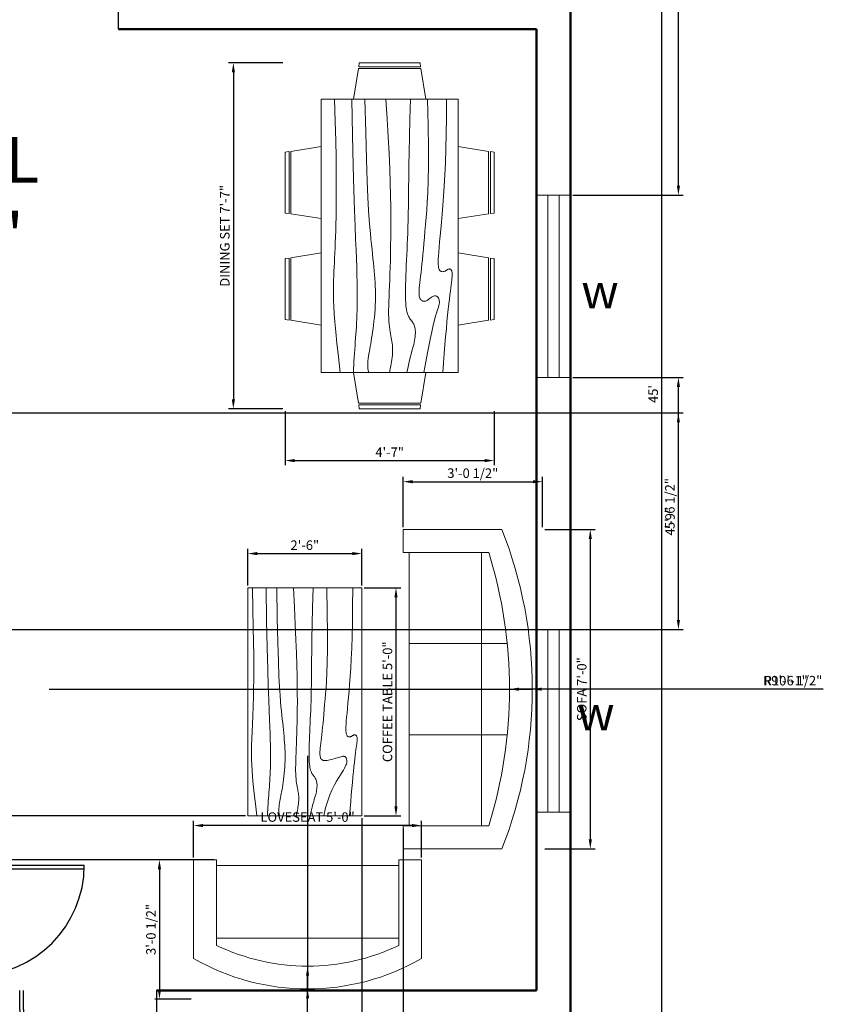
# Model space of a CAD drawing. Units: inches. Extents: x 1962 to 2423, y 2693 to 3296.
# Tile 3 of 4: x 2212 to 2423, y 2833 to 3092. Entities that reach past the tile are written whole.
import ezdxf

# ---------------------------------------------------------------- set-up
doc = ezdxf.new("R2010")
doc.units = ezdxf.units.IN
for name, color, linetype, lineweight in [('A-ANNO-DIMS', 2, 'Continuous', 18), ('A-ANNO-TEXT', 3, 'Continuous', 18), ('A-AREA-IDEN', 7, 'Continuous', 25), ('A-DOOR', 3, 'Continuous', 25), ('A-FURN', 8, 'Continuous', 18), ('A-GLAZ', 4, 'Continuous', 18), ('A-WALL', 7, 'Continuous', 50)]:
    doc.layers.add(name, color=color, linetype=linetype, lineweight=lineweight)
doc.styles.get("Standard").update_dxf_attribs({"font": 'arial.ttf'})
doc.dimstyles.new('ISO-25', dxfattribs={"dimtxt": 2.5, "dimasz": 2.5, "dimexe": 1.25, "dimexo": 0.625, "dimtad": 1, "dimdec": 0, "dimlunit": 3, "dimtxsty": 'Standard', "dimcen": 2.5, "dimadec": 0, "dimazin": 0, "dimtfac": 1, "dimtdec": 0, "dimtmove": 0, "dimatfit": 3, "dimfxl": 1, "dimarcsym": 0})

# ---------------------------------------------------------------- blocks, each defined once
blk = doc.blocks.new('Sofa - Roundback 7 ft.')
for p, q in [((-12.00002, -32.4421), (-12.00003, -6.5971)), ((11.99997, -32.4421), (11.99998, -6.5971)), ((-36.000027, -34), (-36.000027, -11.4696)), ((35.99998, -34), (35.99998, -11.4696)), ((-35.999844, -13.3819), (35.9998, -13.3819)), ((-36.000027, -32.4421), (35.99998, -32.4421))]:
    blk.add_line(p, q)
for points in [[(-36.000027, -34), (-42.000027, -34), (-42.000027, -8)], [(41.99998, -8), (41.99998, -34), (35.99998, -34)]]:
    blk.add_lwpolyline(points)
for centre, radius, start, end in [((0, -114.25), 114.25, 68.43141, 111.5686), ((-0.00001, -127.1968), 121.1968, 72.72033, 107.2797)]:
    blk.add_arc(centre, radius, start, end)
blk = doc.blocks.new('Sofa - Roundback Loveseat 5 ft.')
for p, q in [((0, -32.44198), (0, -5.99998)), ((-24, -33.99998), (-24, -11.46958)), ((24.00004, -33.99998), (24.00004, -11.46958)), ((-23.9998, -13.38178), (23.99986, -13.38178)), ((-24, -32.44198), (24.00004, -32.44198))]:
    blk.add_line(p, q)
for points in [[(-24, -33.99998), (-30, -33.99998), (-30, -7.99998)], [(30.00004, -7.99998), (30.00004, -33.99998), (24.00004, -33.99998)]]:
    blk.add_lwpolyline(points)
for centre, radius, start, end in [((0, -60.24998), 60.24998, 60.13715, 119.8628), ((0, -61.38438), 55.38444, 64.32083, 115.6792)]:
    blk.add_arc(centre, radius, start, end)
blk = doc.blocks.new('Table - Rectangular Woodgrain 60 x 30 in.')
for p, q in [((0, 0), (0, -30)), ((60, 0), (0, 0)), ((60, -30), (60, 0)), ((0, -30), (60, -30))]:
    blk.add_line(p, q)
for points in [[(0, -2.4), (4.8155, -2.418), (9.0302, -2.4688), (12.709, -2.5477), (15.9167, -2.65), (18.7181, -2.7711), (21.1781, -2.9063), (23.3616, -3.0508), (25.3333, -3.2), (27.1477, -3.3495), (28.8172, -3.4958), (30.3437, -3.636), (31.7291, -3.7667), (32.9756, -3.8849), (34.0849, -3.9875), (35.059, -4.0714), (35.9, -4.1334), (36.6114, -4.1711), (37.2041, -4.1854), (37.6906, -4.1779), (38.0833, -4.15), (38.3948, -4.1034), (38.6375, -4.0396), (38.8239, -3.9602), (38.9666, -3.8667), (39.0764, -3.7608), (39.1573, -3.6448), (39.2116, -3.521), (39.2416, -3.3917), (39.2498, -3.2593), (39.2385, -3.1261), (39.21, -2.9944), (39.1666, -2.8667), (39.111, -2.7447), (39.0468, -2.6281), (38.978, -2.5163), (38.9083, -2.4083), (38.8418, -2.3035), (38.7823, -2.201), (38.7337, -2.1001), (38.7, -2), (38.6844, -1.9003), (38.6875, -1.8021), (38.7094, -1.707), (38.75, -1.6167), (38.8094, -1.5326), (38.8875, -1.4563), (38.9844, -1.3893), (39.1, -1.3333), (39.2351, -1.2896), (39.3937, -1.2583), (39.5804, -1.2396), (39.8, -1.2333), (40.057, -1.2396), (40.3562, -1.2583), (40.7023, -1.2896), (41.1, -1.3333), (41.5547, -1.3895), (42.0755, -1.4573), (42.6721, -1.5361), (43.3542, -1.625), (44.1316, -1.7233), (45.014, -1.8302), (46.0114, -1.9449), (47.1333, -2.0667), (48.3862, -2.1947), (49.7625, -2.3281), (51.2513, -2.4663), (52.8416, -2.6083), (54.5226, -2.7535), (56.2833, -2.9011), (58.1127, -3.0501), (60, -3.2)], [(0, -9.2), (6.5759, -9.0858), (11.9385, -9.0365), (16.2527, -9.0418), (19.6833, -9.0917), (22.3952, -9.1759), (24.5531, -9.2844), (26.322, -9.4069), (27.8666, -9.5333), (29.3241, -9.6553), (30.7203, -9.7719), (32.0532, -9.8837), (33.3208, -9.9917), (34.5213, -10.0965), (35.6526, -10.199), (36.7128, -10.2999), (37.7, -10.4), (38.6129, -10.4996), (39.4531, -10.5969), (40.223, -10.6895), (40.925, -10.775), (41.5613, -10.8512), (42.1344, -10.9156), (42.6465, -10.966), (43.1, -11), (43.4976, -11.0158), (43.8437, -11.0136), (44.143, -10.9942), (44.4, -10.9583), (44.6195, -10.9069), (44.8062, -10.8406), (44.9648, -10.7603), (45.1, -10.6667), (45.2155, -10.5598), (45.3114, -10.4365), (45.3871, -10.2929), (45.4416, -10.125), (45.4743, -9.929), (45.4844, -9.7011), (45.4709, -9.4371), (45.4333, -9.1333), (45.3716, -8.7883), (45.2896, -8.4104), (45.1919, -8.0107), (45.0833, -7.6), (44.9685, -7.1893), (44.8521, -6.7896), (44.7388, -6.4117), (44.6333, -6.0667), (44.54, -5.7628), (44.4614, -5.4979), (44.4001, -5.2675), (44.3583, -5.0667), (44.3384, -4.8909), (44.3427, -4.7354), (44.3736, -4.5956), (44.4333, -4.4667), (44.5236, -4.3453), (44.6427, -4.2333), (44.7884, -4.1339), (44.9583, -4.05), (45.1501, -3.9849), (45.3614, -3.9417), (45.59, -3.9234), (45.8333, -3.9333), (46.0915, -3.9749), (46.3734, -4.0531), (46.6906, -4.1736), (47.0542, -4.3417), (47.4756, -4.5629), (47.9661, -4.8427), (48.5372, -5.1866), (49.2, -5.6), (49.9676, -6.0844), (50.8594, -6.625), (51.8965, -7.2031), (53.1, -7.8), (54.491, -8.3969), (56.0906, -8.975), (57.9199, -9.5156), (60, -10)], [(0, -12.8), (5.1847, -12.9322), (9.6213, -13.0323), (13.3963, -13.1059), (16.5958, -13.1583), (19.3063, -13.1952), (21.614, -13.2219), (23.6054, -13.2439), (25.3666, -13.2667), (26.9728, -13.2947), (28.4531, -13.3281), (29.8256, -13.3663), (31.1083, -13.4083), (32.3191, -13.4535), (33.476, -13.501), (34.597, -13.5501), (35.7, -13.6), (36.7984, -13.6497), (37.8875, -13.6979), (38.9578, -13.743), (40, -13.7833), (41.0047, -13.8174), (41.9625, -13.8438), (42.864, -13.8607), (43.7, -13.8667), (44.4631, -13.8604), (45.1552, -13.8417), (45.7801, -13.8104), (46.3416, -13.7667), (46.8439, -13.7104), (47.2906, -13.6417), (47.6858, -13.5604), (48.0333, -13.4667), (48.3375, -13.3608), (48.6042, -13.2448), (48.8396, -13.121), (49.05, -12.9917), (49.2417, -12.8593), (49.4208, -12.7261), (49.5937, -12.5944), (49.7667, -12.4667), (49.9452, -12.3451), (50.1323, -12.2313), (50.3303, -12.1268), (50.5416, -12.0333), (50.7686, -11.9524), (51.0135, -11.8854), (51.2788, -11.8341), (51.5666, -11.8), (51.8785, -11.7843), (52.2116, -11.7865), (52.562, -11.8059), (52.926, -11.8417), (53.2998, -11.8931), (53.6795, -11.9594), (54.0614, -12.0397), (54.4416, -12.1333), (54.8223, -12.2401), (55.2293, -12.3625), (55.6942, -12.5037), (56.2489, -12.6667), (56.9251, -12.8547), (57.7545, -13.0708), (58.7689, -13.3182), (60, -13.6)], [(0, -18), (5.124, -17.7273), (9.6609, -17.5057), (13.6705, -17.3303), (17.2125, -17.1958), (20.3467, -17.0973), (23.1328, -17.0297), (25.6307, -16.9878), (27.9, -16.9667), (29.9928, -16.9617), (31.9302, -16.9703), (33.7254, -16.9907), (35.3917, -17.0208), (36.9423, -17.0588), (38.3906, -17.1026), (39.7499, -17.1503), (41.0333, -17.2), (42.2519, -17.2496), (43.4073, -17.2969), (44.4986, -17.3395), (45.525, -17.375), (46.4858, -17.4012), (47.3802, -17.4156), (48.2074, -17.416), (48.9667, -17.4), (49.6583, -17.3662), (50.2872, -17.3167), (50.8595, -17.2547), (51.3812, -17.1833), (51.8584, -17.1057), (52.2971, -17.025), (52.7034, -16.9443), (53.0833, -16.8667), (53.443, -16.7951), (53.789, -16.7313), (54.128, -16.6768), (54.4666, -16.6334), (54.8115, -16.6024), (55.1693, -16.5854), (55.5465, -16.5841), (55.95, -16.6), (56.3828, -16.6337), (56.8346, -16.6823), (57.2915, -16.7418), (57.7396, -16.8084), (58.165, -16.878), (58.5539, -16.9469), (58.8924, -17.0111), (59.1666, -17.0667), (59.3679, -17.1107), (59.5078, -17.1438), (59.6032, -17.1675), (59.6708, -17.1833), (59.7275, -17.193), (59.7901, -17.1979), (59.8753, -17.1998), (60, -17.2)], [(0, -22.4), (8.0098, -22.2501), (14.4094, -22.1011), (19.4168, -21.9535), (23.25, -21.8083), (26.1269, -21.6663), (28.2656, -21.5281), (29.884, -21.3947), (31.2, -21.2667), (32.3967, -21.1448), (33.5172, -21.0292), (34.5697, -20.9198), (35.5625, -20.8167), (36.5037, -20.7198), (37.4015, -20.6292), (38.2642, -20.5448), (39.1, -20.4667), (39.9164, -20.3951), (40.7187, -20.3313), (41.5117, -20.2768), (42.3, -20.2333), (43.0883, -20.2024), (43.8812, -20.1854), (44.6836, -20.1841), (45.5, -20.2), (46.3328, -20.234), (47.1747, -20.2844), (48.0163, -20.3488), (48.8479, -20.425), (49.66, -20.5106), (50.4429, -20.6031), (51.1872, -20.7004), (51.8833, -20.8), (52.5246, -20.8999), (53.1166, -20.9995), (53.6681, -21.0983), (54.1875, -21.1958), (54.6834, -21.2919), (55.1646, -21.3859), (55.6394, -21.4777), (56.1167, -21.5667), (56.6028, -21.6515), (57.0961, -21.7266), (57.5929, -21.7852), (58.0896, -21.8208), (58.5823, -21.8268), (59.0674, -21.7964), (59.5412, -21.723), (60, -21.6)], [(0, -25.2), (8.6355, -25.0504), (15.7026, -24.9031), (21.4049, -24.7606), (25.9458, -24.625), (29.529, -24.4988), (32.3578, -24.3844), (34.6359, -24.284), (36.5667, -24.2), (38.3213, -24.1341), (39.9417, -24.0854), (41.437, -24.0523), (42.8167, -24.0333), (44.0901, -24.0268), (45.2667, -24.0313), (46.3557, -24.0451), (47.3667, -24.0667), (48.309, -24.0947), (49.1928, -24.1287), (50.0284, -24.168), (50.826, -24.2125), (51.5959, -24.2617), (52.3483, -24.3151), (53.0935, -24.3725), (53.8417, -24.4334), (54.6009, -24.497), (55.3699, -24.561), (56.1454, -24.6226), (56.9239, -24.6792), (57.7021, -24.7279), (58.4764, -24.7662), (59.2435, -24.7911), (60, -24.8)], [(0, -28.8), (5.6867, -28.6681), (10.45, -28.5698), (14.407, -28.5012), (17.675, -28.4584), (20.3711, -28.4374), (22.6125, -28.4344), (24.5164, -28.4455), (26.2, -28.4667), (27.762, -28.4947), (29.2276, -28.5281), (30.6033, -28.5663), (31.8958, -28.6084), (33.1118, -28.6535), (34.2578, -28.7011), (35.3405, -28.7501), (36.3666, -28.8), (37.3443, -28.8497), (38.288, -28.8974), (39.2137, -28.9412), (40.1375, -28.9792), (41.0753, -29.0093), (42.0432, -29.0297), (43.0572, -29.0384), (44.1333, -29.0333), (45.2936, -29.0114), (46.5843, -28.9641), (48.0579, -28.8816), (49.7666, -28.7542), (51.7629, -28.5721), (54.0989, -28.3255), (56.8272, -28.0048), (60, -27.6)]]:
    blk.add_lwpolyline(points)
blk = doc.blocks.new('Dining Set - 36 x 72 in.')
for p, q in [((-22.2343, 26.00059), (-23.4847, 17.99762)), ((-22.2304, 26), (-5.7608, 26)), ((-22, 27.5), (-22.1562, 26.50042)), ((-5.8416, 26.5), (-22.1534, 26.5)), ((-22, 27.5), (-6, 27.5)), ((-5.8437, 26.49966), (-6, 27.5)), ((-4.5152, 17.99762), (-5.7655, 25.99926)), ((5.7657, 26.00059), (4.5153, 17.99762)), ((5.7696, 26), (22.2392, 26)), ((6, 27.5), (5.8438, 26.50042)), ((22.1584, 26.5), (5.8466, 26.5)), ((6, 27.5), (22, 27.5)), ((22.1563, 26.49966), (22, 27.5)), ((23.4848, 17.99762), (22.2345, 25.99926)), ((36, 18), (-36, 18)), ((-36, 18), (-36, -18)), ((36, -18), (36, 18)), ((-45.5, 8), (-44.5004, 8.15617)), ((-45.5, 8), (-45.5, -8)), ((-44.5, -8.15843), (-44.5, 8.15338)), ((-44.0006, 8.23428), (-35.9976, 9.48474)), ((-44, 8.23041), (-44, -8.23915)), ((44.0006, 8.23428), (35.9976, 9.48474)), ((44, 8.23041), (44, -8.23915)), ((44.5, -8.15843), (44.5, 8.15338)), ((45.5, 8), (44.5005, 8.15617)), ((45.5, 8), (45.5, -8)), ((-44.4997, -8.15631), (-45.5, -8)), ((-35.9976, -9.48476), (-43.9993, -8.2345)), ((35.9976, -9.48476), (43.9993, -8.2345)), ((44.4997, -8.15631), (45.5, -8)), ((-36, -18), (36, -18)), ((-22.2343, -26.0006), (-23.4847, -17.99762)), ((-4.5152, -17.99762), (-5.7655, -25.99928)), ((5.7657, -26.0006), (4.5153, -17.99762)), ((23.4848, -17.99762), (22.2345, -25.99928)), ((-22.2304, -26), (-5.7608, -26)), ((-22, -27.5), (-22.1562, -26.50044)), ((-5.8416, -26.5), (-22.1534, -26.5)), ((-22, -27.5), (-6, -27.5)), ((-5.8437, -26.49967), (-6, -27.5)), ((5.7696, -26), (22.2392, -26)), ((6, -27.5), (5.8438, -26.50044)), ((22.1584, -26.5), (5.8466, -26.5)), ((6, -27.5), (22, -27.5)), ((22.1563, -26.49967), (22, -27.5))]:
    blk.add_line(p, q)
for points in [[(-36, 15), (-31.1772, 14.97754), (-26.8079, 14.91406), (-22.8538, 14.81543), (-19.276, 14.6875), (-16.0362, 14.53613), (-13.0957, 14.36718), (-10.4159, 14.18652), (-7.9583, 14), (-5.6904, 13.81315), (-3.6035, 13.63021), (-1.6954, 13.45508), (0.0365, 13.29166), (1.5945, 13.14388), (2.9811, 13.01562), (4.1988, 12.9108), (5.25, 12.83333), (6.1393, 12.78613), (6.8802, 12.76823), (7.4883, 12.77767), (7.9792, 12.8125), (8.3685, 12.87077), (8.6719, 12.95052), (8.9049, 13.0498), (9.0833, 13.16666), (9.2205, 13.29899), (9.3216, 13.44401), (9.3895, 13.59879), (9.4271, 13.76041), (9.4373, 13.92594), (9.4232, 14.09245), (9.3875, 14.257), (9.3333, 14.41666), (9.2638, 14.56917), (9.1836, 14.71484), (9.0975, 14.85465), (9.0104, 14.98958), (8.9272, 15.1206), (8.8529, 15.2487), (8.7922, 15.37483), (8.75, 15.5), (8.7305, 15.62467), (8.7344, 15.74739), (8.7617, 15.86621), (8.8125, 15.97916), (8.8867, 16.08431), (8.9844, 16.17968), (9.1055, 16.26334), (9.25, 16.33333), (9.4189, 16.38802), (9.6172, 16.42708), (9.8506, 16.45052), (10.125, 16.45833), (10.4463, 16.45052), (10.8203, 16.42708), (11.2529, 16.38802), (11.75, 16.33333), (12.3184, 16.26318), (12.9694, 16.17838), (13.7151, 16.07991), (14.5677, 15.96875), (15.5395, 15.84586), (16.6426, 15.71224), (17.8893, 15.56884), (19.2917, 15.41666), (20.859, 15.25667), (22.5879, 15.08984), (24.4721, 14.91715), (26.5052, 14.73958), (28.6809, 14.5581), (30.9929, 14.3737), (33.4347, 14.18733), (36, 14)], [(-36, 10), (-28.9766, 10.14274), (-23.1725, 10.20442), (-18.4241, 10.19775), (-14.5677, 10.13541), (-11.4399, 10.03011), (-8.877, 9.89453), (-6.7154, 9.74137), (-4.7917, 9.58333), (-2.9698, 9.43082), (-1.2246, 9.28515), (0.4415, 9.14534), (2.026, 9.01041), (3.5266, 8.87939), (4.9408, 8.7513), (6.266, 8.62516), (7.5, 8.5), (8.6411, 8.37549), (9.6914, 8.2539), (10.6538, 8.13818), (11.5312, 8.03125), (12.3267, 7.93603), (13.043, 7.85547), (13.6831, 7.79248), (14.25, 7.75), (14.7471, 7.7303), (15.1797, 7.73307), (15.5537, 7.75732), (15.875, 7.80208), (16.1494, 7.86637), (16.3828, 7.94922), (16.5811, 8.04964), (16.75, 8.16666), (16.8944, 8.29915), (17.0143, 8.44531), (17.1089, 8.60319), (17.1771, 8.77083), (17.218, 8.94629), (17.2305, 9.1276), (17.2137, 9.31282), (17.1667, 9.5), (17.0895, 9.6875), (16.987, 9.875), (16.8649, 10.0625), (16.7292, 10.25), (16.5856, 10.4375), (16.4401, 10.625), (16.2985, 10.8125), (16.1667, 11), (16.05, 11.18733), (15.9518, 11.3737), (15.8752, 11.5581), (15.8229, 11.73958), (15.798, 11.91715), (15.8034, 12.08984), (15.842, 12.25667), (15.9167, 12.41666), (16.0295, 12.56836), (16.1784, 12.70833), (16.3605, 12.83268), (16.5729, 12.9375), (16.8127, 13.01888), (17.0768, 13.07291), (17.3625, 13.0957), (17.6667, 13.08333), (17.9894, 13.03312), (18.3418, 12.94726), (18.7382, 12.82918), (19.1927, 12.68229), (19.7195, 12.51001), (20.3327, 12.31575), (21.0465, 12.10294), (21.875, 11.875), (22.8357, 11.63354), (23.959, 11.37304), (25.2786, 11.08618), (26.8282, 10.76562), (28.6414, 10.40405), (30.752, 9.99414), (33.1936, 9.52856), (36, 9)], [(-36, 5.5), (-30.7157, 5.3348), (-26.069, 5.20963), (-21.9946, 5.11767), (-18.4271, 5.05208), (-15.3009, 5.00602), (-12.5508, 4.97265), (-10.1112, 4.94515), (-7.9167, 4.91666), (-5.909, 4.88167), (-4.0586, 4.83984), (-2.3429, 4.79215), (-0.7396, 4.73958), (0.7739, 4.6831), (2.22, 4.6237), (3.6213, 4.56233), (5, 4.5), (6.373, 4.43782), (7.7344, 4.3776), (9.0723, 4.32129), (10.375, 4.27083), (11.6309, 4.22819), (12.8281, 4.19531), (13.9551, 4.17415), (15, 4.16666), (15.954, 4.17448), (16.819, 4.19791), (17.6001, 4.23698), (18.3021, 4.29166), (18.9299, 4.36198), (19.4883, 4.44791), (19.9823, 4.54948), (20.4167, 4.66666), (20.7969, 4.79899), (21.1302, 4.94401), (21.4245, 5.09879), (21.6875, 5.26041), (21.9271, 5.42594), (22.1511, 5.59245), (22.3672, 5.757), (22.5834, 5.91666), (22.8065, 6.06868), (23.0404, 6.21093), (23.2879, 6.34147), (23.5521, 6.45833), (23.8358, 6.55957), (24.142, 6.64323), (24.4735, 6.70735), (24.8334, 6.75), (25.2235, 6.76969), (25.642, 6.76692), (26.0858, 6.74267), (26.5521, 6.69791), (27.0379, 6.63362), (27.5404, 6.55078), (28.0565, 6.45036), (28.5834, 6.33333), (29.1242, 6.19987), (29.7071, 6.04687), (30.3661, 5.87044), (31.1354, 5.66666), (32.0493, 5.43164), (33.142, 5.16146), (34.4475, 4.85221), (36, 4.5)], [(-36, -1), (-30.7915, -0.6591), (-26.0195, -0.38216), (-21.6519, -0.16284), (-17.6563, 0.00521), (-14.0005, 0.12833), (-10.6523, 0.21289), (-7.5796, 0.26522), (-4.75, 0.29166), (-2.134, 0.29793), (0.2878, 0.28711), (2.5317, 0.26163), (4.6146, 0.22396), (6.5529, 0.17651), (8.3633, 0.12174), (10.0623, 0.06209), (11.6667, 0), (13.1899, -0.06201), (14.6341, -0.1211), (15.9982, -0.17432), (17.2813, -0.21875), (18.4823, -0.25147), (19.6003, -0.26953), (20.6343, -0.27002), (21.5834, -0.25), (22.4481, -0.20768), (23.2357, -0.14584), (23.9549, -0.06836), (24.6146, 0.02083), (25.2235, 0.11784), (25.7904, 0.21875), (26.3241, 0.31966), (26.8334, 0.41666), (27.3265, 0.50618), (27.8099, 0.58593), (28.2894, 0.65397), (28.7709, 0.70833), (29.2601, 0.74707), (29.763, 0.76823), (30.2855, 0.76985), (30.8334, 0.75), (31.4088, 0.70784), (31.9994, 0.64713), (32.589, 0.57275), (33.1615, 0.48958), (33.7008, 0.4025), (34.1908, 0.3164), (34.6153, 0.23616), (34.9584, 0.16666), (35.2099, 0.11165), (35.3848, 0.07031), (35.504, 0.04069), (35.5886, 0.02083), (35.6594, 0.00879), (35.7377, 0.0026), (35.8442, 0.00032), (36, 0)], [(-36, -6.5), (-27.1843, -6.31267), (-20.084, -6.1263), (-14.469, -5.9419), (-10.1094, -5.76042), (-6.7752, -5.58285), (-4.2363, -5.41016), (-2.2629, -5.24333), (-0.625, -5.08334), (0.8708, -4.93099), (2.2715, -4.78646), (3.5872, -4.64974), (4.8281, -4.52084), (6.0046, -4.39974), (7.127, -4.28646), (8.2053, -4.18099), (9.25, -4.08334), (10.2705, -3.99382), (11.2734, -3.91407), (12.2647, -3.84603), (13.25, -3.79167), (14.2354, -3.75293), (15.2266, -3.73177), (16.2295, -3.73015), (17.25, -3.75), (18.2912, -3.79248), (19.3451, -3.85547), (20.4009, -3.93604), (21.4479, -4.03125), (22.4754, -4.13819), (23.4727, -4.25391), (24.4289, -4.37549), (25.3334, -4.5), (26.1785, -4.62492), (26.9694, -4.74935), (27.7145, -4.87281), (28.4219, -4.99479), (29.1, -5.11483), (29.7572, -5.23242), (30.4016, -5.34709), (31.0417, -5.45834), (31.6837, -5.56437), (32.3262, -5.65821), (32.9658, -5.73153), (33.599, -5.77604), (34.2224, -5.78345), (34.8327, -5.74545), (35.4264, -5.65373), (36, -5.5)], [(-36, -10), (-26.4022, -9.81299), (-18.4675, -9.62891), (-11.9839, -9.45069), (-6.7396, -9.28125), (-2.5226, -9.12354), (0.8789, -8.98047), (3.6769, -8.85498), (6.0833, -8.75), (8.2767, -8.66765), (10.3021, -8.60677), (12.1712, -8.56543), (13.8958, -8.54167), (15.4876, -8.53353), (16.9583, -8.53907), (18.3197, -8.55632), (19.5834, -8.58334), (20.7616, -8.61841), (21.8685, -8.66081), (22.9188, -8.71004), (23.9271, -8.76563), (24.9081, -8.82707), (25.8763, -8.89388), (26.8465, -8.96558), (27.8334, -9.04167), (28.8474, -9.12118), (29.8828, -9.20117), (30.93, -9.27824), (31.9792, -9.34896), (33.0205, -9.40991), (34.0443, -9.45768), (35.0407, -9.48885), (36, -9.5)], [(-36, -14.5), (-30.0881, -14.33513), (-25.0332, -14.21224), (-20.7312, -14.12647), (-17.0781, -14.07292), (-13.97, -14.04671), (-11.3027, -14.04297), (-8.9724, -14.05681), (-6.875, -14.08334), (-4.9224, -14.11833), (-3.0905, -14.16016), (-1.3709, -14.20785), (0.2448, -14.26042), (1.7647, -14.3169), (3.1973, -14.3763), (4.5507, -14.43767), (5.8333, -14.5), (7.0554, -14.5621), (8.235, -14.62175), (9.3922, -14.67652), (10.5469, -14.72396), (11.7192, -14.76164), (12.929, -14.78711), (14.1965, -14.79794), (15.5417, -14.79167), (16.9933, -14.76424), (18.6152, -14.70508), (20.4804, -14.60197), (22.6615, -14.44271), (25.2312, -14.21509), (28.2624, -13.9069), (31.8277, -13.50594), (36, -13)]]:
    blk.add_lwpolyline(points)
blk = doc.blocks.new('*D13')
at = {"layer": 'A-ANNO-DIMS', "color": 0, "lineweight": -2, "transparency": 16777216}
for p, q in [((2357.16, 3263.59), (2381.77, 3263.59)), ((2380.52, 3261.09), (2380.52, 2726.09)), ((2357.16, 2723.59), (2381.77, 2723.59))]:
    blk.add_line(p, q, dxfattribs=at)
at = {"layer": 'A-ANNO-DIMS', "color": 0, "transparency": 16777216}
for points in [[(2380.1, 3261.09), (2380.94, 3261.09), (2380.52, 3263.59)], [(2380.1, 2726.09), (2380.94, 2726.09), (2380.52, 2723.59)]]:
    blk.add_solid(points, dxfattribs=at)
at = {"layer": 'Defpoints', "color": 0, "transparency": 16777216}
for p in [(2356.54, 3263.59), (2356.54, 2723.59), (2380.52, 2723.59)]:
    blk.add_point(p, dxfattribs=at)
at = {"layer": 'A-ANNO-DIMS', "color": 0, "transparency": 16777216, "insert": (2378.62, 2993.59), "char_height": 2.5, "attachment_point": 5, "rotation": 90}
blk.add_mtext("45'", dxfattribs=at)
blk = doc.blocks.new('DOOR-SWING-36IN')
for p, q in [((0, 5), (0, 41)), ((1, 5), (1, 41)), ((0, 5), (0, 0)), ((1, 5), (1, 0)), ((36, 0), (36, 5))]:
    blk.add_line(p, q)
blk.add_arc((0, 5), 36, 0, 90)
blk = doc.blocks.new('DOOR-SWING-29IN')
for p, q in [((0, 5), (0, 34)), ((1, 5), (1, 34)), ((0, 5), (0, 0)), ((1, 5), (1, 0)), ((29, 0), (29, 5))]:
    blk.add_line(p, q)
blk.add_arc((0, 5), 29, 0, 90)
blk = doc.blocks.new('WINDOW-48IN')
for p, q in [((0, 48), (0, 0)), ((9, 48), (0, 48)), ((3, 48), (3, 0)), ((6, 0), (6, 48)), ((9, 0), (9, 48)), ((0, 0), (9, 0))]:
    blk.add_line(p, q)
blk = doc.blocks.new('*D42')
at = {"layer": 'A-ANNO-DIMS', "color": 0, "lineweight": -2, "transparency": 16777216}
for p, q in [((2349.77, 2957.9), (2362.99, 2957.9)), ((2361.74, 2955.4), (2361.74, 2876.4)), ((2349.77, 2873.9), (2362.99, 2873.9))]:
    blk.add_line(p, q, dxfattribs=at)
at = {"layer": 'A-ANNO-DIMS', "color": 0, "transparency": 16777216}
for points in [[(2361.32, 2955.4), (2362.16, 2955.4), (2361.74, 2957.9)], [(2361.32, 2876.4), (2362.16, 2876.4), (2361.74, 2873.9)]]:
    blk.add_solid(points, dxfattribs=at)
at = {"layer": 'Defpoints', "color": 0, "transparency": 16777216}
for p in [(2349.14, 2957.9), (2349.14, 2873.9), (2361.74, 2873.9)]:
    blk.add_point(p, dxfattribs=at)
at = {"layer": 'A-ANNO-DIMS', "color": 0, "transparency": 16777216, "insert": (2359.82, 2915.9), "char_height": 2.5, "attachment_point": 5, "rotation": 90}
blk.add_mtext('SOFA 7\'-0"', dxfattribs=at)
blk = doc.blocks.new('*D43')
at = {"layer": 'A-ANNO-DIMS', "color": 0, "lineweight": -2, "transparency": 16777216}
for p, q in [((2312.47, 2958.52), (2312.47, 2971.75)), ((2314.97, 2970.5), (2346.64, 2970.5)), ((2349.14, 2958.52), (2349.14, 2971.75))]:
    blk.add_line(p, q, dxfattribs=at)
at = {"layer": 'A-ANNO-DIMS', "color": 0, "transparency": 16777216}
for points in [[(2314.97, 2970.91), (2314.97, 2970.08), (2312.47, 2970.5)], [(2346.64, 2970.91), (2346.64, 2970.08), (2349.14, 2970.5)]]:
    blk.add_solid(points, dxfattribs=at)
at = {"layer": 'Defpoints', "color": 0, "transparency": 16777216}
for p in [(2349.14, 2970.5), (2312.47, 2957.9), (2349.14, 2957.9)]:
    blk.add_point(p, dxfattribs=at)
at = {"layer": 'A-ANNO-DIMS', "color": 0, "transparency": 16777216, "insert": (2330.81, 2972.42), "char_height": 2.5, "attachment_point": 5}
blk.add_mtext('3\'-0 1/2"', dxfattribs=at)
blk = doc.blocks.new('*D44')
at = {"layer": 'A-ANNO-DIMS', "color": 0, "lineweight": -2, "transparency": 16777216}
for p, q in [((2257.33, 2871.63), (2257.33, 2881.26)), ((2314.83, 2880.01), (2259.83, 2880.01)), ((2317.33, 2871.63), (2317.33, 2881.26))]:
    blk.add_line(p, q, dxfattribs=at)
at = {"layer": 'A-ANNO-DIMS', "color": 0, "transparency": 16777216}
for points in [[(2259.83, 2880.42), (2259.83, 2879.59), (2257.33, 2880.01)], [(2314.83, 2880.42), (2314.83, 2879.59), (2317.33, 2880.01)]]:
    blk.add_solid(points, dxfattribs=at)
at = {"layer": 'Defpoints', "color": 0, "transparency": 16777216}
for p in [(2257.33, 2880.01), (2257.33, 2871.01), (2317.33, 2871.01)]:
    blk.add_point(p, dxfattribs=at)
at = {"layer": 'A-ANNO-DIMS', "color": 0, "transparency": 16777216, "insert": (2287.33, 2881.92), "char_height": 2.5, "attachment_point": 5}
blk.add_mtext('LOVESEAT 5\'-0"', dxfattribs=at)
blk = doc.blocks.new('*D45')
at = {"layer": 'A-ANNO-DIMS', "color": 0, "lineweight": -2, "transparency": 16777216}
for p, q in [((2256.7, 2871.01), (2247.08, 2871.01)), ((2248.33, 2868.51), (2248.33, 2836.84)), ((2256.7, 2834.34), (2247.08, 2834.34))]:
    blk.add_line(p, q, dxfattribs=at)
at = {"layer": 'A-ANNO-DIMS', "color": 0, "transparency": 16777216}
for points in [[(2247.91, 2868.51), (2248.74, 2868.51), (2248.33, 2871.01)], [(2247.91, 2836.84), (2248.74, 2836.84), (2248.33, 2834.34)]]:
    blk.add_solid(points, dxfattribs=at)
at = {"layer": 'Defpoints', "color": 0, "transparency": 16777216}
for p in [(2257.33, 2871.01), (2248.33, 2834.34), (2257.33, 2834.34)]:
    blk.add_point(p, dxfattribs=at)
at = {"layer": 'A-ANNO-DIMS', "color": 0, "transparency": 16777216, "insert": (2246.41, 2852.67), "char_height": 2.5, "attachment_point": 5, "rotation": 90}
blk.add_mtext('3\'-0 1/2"', dxfattribs=at)
blk = doc.blocks.new('*D46')
at = {"layer": 'A-ANNO-DIMS', "color": 0, "lineweight": -2, "transparency": 16777216}
for p, q in [((2302.21, 2942.58), (2311.84, 2942.58)), ((2310.59, 2940.08), (2310.59, 2885.08)), ((2302.21, 2882.58), (2311.84, 2882.58))]:
    blk.add_line(p, q, dxfattribs=at)
at = {"layer": 'A-ANNO-DIMS', "color": 0, "transparency": 16777216}
for points in [[(2310.17, 2940.08), (2311, 2940.08), (2310.59, 2942.58)], [(2310.17, 2885.08), (2311, 2885.08), (2310.59, 2882.58)]]:
    blk.add_solid(points, dxfattribs=at)
at = {"layer": 'Defpoints', "color": 0, "transparency": 16777216}
for p in [(2301.59, 2942.58), (2301.59, 2882.58), (2310.59, 2882.58)]:
    blk.add_point(p, dxfattribs=at)
at = {"layer": 'A-ANNO-DIMS', "color": 0, "transparency": 16777216, "insert": (2308.67, 2912.58), "char_height": 2.5, "attachment_point": 5, "rotation": 90}
blk.add_mtext('COFFEE TABLE 5\'-0"', dxfattribs=at)
blk = doc.blocks.new('*D47')
at = {"layer": 'A-ANNO-DIMS', "color": 0, "lineweight": -2, "transparency": 16777216}
for p, q in [((2271.59, 2943.2), (2271.59, 2952.83)), ((2274.09, 2951.58), (2299.09, 2951.58)), ((2301.59, 2943.2), (2301.59, 2952.83))]:
    blk.add_line(p, q, dxfattribs=at)
at = {"layer": 'A-ANNO-DIMS', "color": 0, "transparency": 16777216}
for points in [[(2274.09, 2952), (2274.09, 2951.16), (2271.59, 2951.58)], [(2299.09, 2952), (2299.09, 2951.16), (2301.59, 2951.58)]]:
    blk.add_solid(points, dxfattribs=at)
at = {"layer": 'Defpoints', "color": 0, "transparency": 16777216}
for p in [(2301.59, 2951.58), (2271.59, 2942.58), (2301.59, 2942.58)]:
    blk.add_point(p, dxfattribs=at)
at = {"layer": 'A-ANNO-DIMS', "color": 0, "transparency": 16777216, "insert": (2286.59, 2953.48), "char_height": 2.5, "attachment_point": 5}
blk.add_mtext('2\'-6"', dxfattribs=at)
blk = doc.blocks.new('*D50')
at = {"layer": 'A-ANNO-DIMS', "color": 0, "lineweight": -2, "transparency": 16777216}
for p, q in [((2280.81, 3080.71), (2266.53, 3080.71)), ((2267.78, 3078.21), (2267.78, 2992.21)), ((2280.81, 2989.71), (2266.53, 2989.71))]:
    blk.add_line(p, q, dxfattribs=at)
at = {"layer": 'A-ANNO-DIMS', "color": 0, "transparency": 16777216}
for points in [[(2267.37, 3078.21), (2268.2, 3078.21), (2267.78, 3080.71)], [(2267.37, 2992.21), (2268.2, 2992.21), (2267.78, 2989.71)]]:
    blk.add_solid(points, dxfattribs=at)
at = {"layer": 'Defpoints', "color": 0, "transparency": 16777216}
for p in [(2281.43, 3080.71), (2267.78, 2989.71), (2281.43, 2989.71)]:
    blk.add_point(p, dxfattribs=at)
at = {"layer": 'A-ANNO-DIMS', "color": 0, "transparency": 16777216, "insert": (2265.86, 3035.21), "char_height": 2.5, "attachment_point": 5, "rotation": 90}
blk.add_mtext('DINING SET 7\'-7"', dxfattribs=at)
blk = doc.blocks.new('*D51')
at = {"layer": 'A-ANNO-DIMS', "color": 0, "lineweight": -2, "transparency": 16777216}
for p, q in [((2281.43, 2989.08), (2281.43, 2974.81)), ((2336.43, 2989.08), (2336.43, 2974.81)), ((2283.93, 2976.06), (2333.93, 2976.06))]:
    blk.add_line(p, q, dxfattribs=at)
at = {"layer": 'A-ANNO-DIMS', "color": 0, "transparency": 16777216}
for points in [[(2283.93, 2976.47), (2283.93, 2975.64), (2281.43, 2976.06)], [(2333.93, 2976.47), (2333.93, 2975.64), (2336.43, 2976.06)]]:
    blk.add_solid(points, dxfattribs=at)
at = {"layer": 'Defpoints', "color": 0, "transparency": 16777216}
for p in [(2281.43, 2989.71), (2336.43, 2989.71), (2336.43, 2976.06)]:
    blk.add_point(p, dxfattribs=at)
at = {"layer": 'A-ANNO-DIMS', "color": 0, "transparency": 16777216, "insert": (2308.93, 2977.93), "char_height": 2.5, "attachment_point": 5}
blk.add_mtext('4\'-7"', dxfattribs=at)
blk = doc.blocks.new('*D52')
at = {"layer": 'A-ANNO-DIMS', "color": 0, "lineweight": -2, "transparency": 16777216}
for p, q in [((2195.16, 2988.59), (2386.19, 2988.59)), ((2384.94, 2934.09), (2384.94, 2986.09)), ((2195.16, 2931.59), (2386.19, 2931.59))]:
    blk.add_line(p, q, dxfattribs=at)
at = {"layer": 'A-ANNO-DIMS', "color": 0, "transparency": 16777216}
for points in [[(2384.52, 2986.09), (2385.35, 2986.09), (2384.94, 2988.59)], [(2384.52, 2934.09), (2385.35, 2934.09), (2384.94, 2931.59)]]:
    blk.add_solid(points, dxfattribs=at)
at = {"layer": 'Defpoints', "color": 0, "transparency": 16777216}
for p in [(2194.54, 2988.59), (2384.94, 2988.59), (2194.54, 2931.59)]:
    blk.add_point(p, dxfattribs=at)
at = {"layer": 'A-ANNO-DIMS', "color": 0, "transparency": 16777216, "insert": (2383.04, 2960.09), "char_height": 2.5, "attachment_point": 5, "rotation": 90}
blk.add_mtext('4\'-9"', dxfattribs=at)
blk = doc.blocks.new('*D60')
at = {"layer": 'A-ANNO-DIMS', "color": 0, "lineweight": -2, "transparency": 16777216}
for p, q in [((2357.16, 3169.58), (2386.19, 3169.58)), ((2384.94, 3048.42), (2384.94, 3167.08)), ((2357.16, 3045.92), (2386.19, 3045.92))]:
    blk.add_line(p, q, dxfattribs=at)
at = {"layer": 'A-ANNO-DIMS', "color": 0, "transparency": 16777216}
for points in [[(2384.52, 3167.08), (2385.35, 3167.08), (2384.94, 3169.58)], [(2384.52, 3048.42), (2385.35, 3048.42), (2384.94, 3045.92)]]:
    blk.add_solid(points, dxfattribs=at)
at = {"layer": 'Defpoints', "color": 0, "transparency": 16777216}
for p in [(2356.54, 3169.58), (2384.94, 3169.58), (2356.54, 3045.92)]:
    blk.add_point(p, dxfattribs=at)
at = {"layer": 'A-ANNO-DIMS', "color": 0, "transparency": 16777216, "insert": (2383.02, 3107.75), "char_height": 2.5, "attachment_point": 5, "rotation": 90}
blk.add_mtext('10\'-3 1/2"', dxfattribs=at)
blk = doc.blocks.new('*D61')
at = {"layer": 'A-ANNO-DIMS', "color": 0, "lineweight": -2, "transparency": 16777216}
for p, q in [((2357.16, 2997.92), (2386.19, 2997.92)), ((2384.94, 2934.07), (2384.94, 2995.42)), ((2357.16, 2931.57), (2386.19, 2931.57))]:
    blk.add_line(p, q, dxfattribs=at)
at = {"layer": 'A-ANNO-DIMS', "color": 0, "transparency": 16777216}
for points in [[(2384.52, 2995.42), (2385.35, 2995.42), (2384.94, 2997.92)], [(2384.52, 2934.07), (2385.35, 2934.07), (2384.94, 2931.57)]]:
    blk.add_solid(points, dxfattribs=at)
at = {"layer": 'Defpoints', "color": 0, "transparency": 16777216}
for p in [(2356.54, 2997.92), (2384.94, 2997.92), (2356.54, 2931.57)]:
    blk.add_point(p, dxfattribs=at)
at = {"layer": 'A-ANNO-DIMS', "color": 0, "transparency": 16777216, "insert": (2383.02, 2964.75), "char_height": 2.5, "attachment_point": 5, "rotation": 90}
blk.add_mtext('5\'-6 1/2"', dxfattribs=at)
blk = doc.blocks.new('*D65')
at = {"layer": 'A-ANNO-DIMS', "color": 0, "lineweight": -2, "transparency": 16777216}
for p, q in [((2301.59, 2881.95), (2301.59, 2693.94)), ((2312.47, 2879.27), (2312.47, 2693.94)), ((2304.09, 2695.19), (2309.97, 2695.19))]:
    blk.add_line(p, q, dxfattribs=at)
at = {"layer": 'A-ANNO-DIMS', "color": 0, "transparency": 16777216}
for points in [[(2304.09, 2695.61), (2304.09, 2694.77), (2301.59, 2695.19)], [(2309.97, 2695.61), (2309.97, 2694.77), (2312.47, 2695.19)]]:
    blk.add_solid(points, dxfattribs=at)
at = {"layer": 'Defpoints', "color": 0, "transparency": 16777216}
for p in [(2301.59, 2882.58), (2312.47, 2879.9), (2312.47, 2695.19)]:
    blk.add_point(p, dxfattribs=at)
at = {"layer": 'A-ANNO-DIMS', "color": 0, "transparency": 16777216, "insert": (2307.03, 2697.09), "char_height": 2.5, "attachment_point": 5}
blk.add_mtext('0\'-11"', dxfattribs=at)
blk = doc.blocks.new('*D66')
at = {"layer": 'A-ANNO-DIMS', "color": 0, "lineweight": -2, "transparency": 16777216}
for p, q in [((2270.96, 2882.58), (1966.89, 2882.58)), ((1968.14, 2880.08), (1968.14, 2873.51)), ((2262.7, 2871.01), (1966.89, 2871.01)), ((1968.14, 2871.01), (1968.14, 2852.84))]:
    blk.add_line(p, q, dxfattribs=at)
at = {"layer": 'A-ANNO-DIMS', "color": 0, "transparency": 16777216}
for points in [[(1967.72, 2880.08), (1968.55, 2880.08), (1968.14, 2882.58)], [(1967.72, 2873.51), (1968.55, 2873.51), (1968.14, 2871.01)]]:
    blk.add_solid(points, dxfattribs=at)
at = {"layer": 'Defpoints', "color": 0, "transparency": 16777216}
for p in [(2271.59, 2882.58), (1968.14, 2871.01), (2263.33, 2871.01)]:
    blk.add_point(p, dxfattribs=at)
at = {"layer": 'A-ANNO-DIMS', "color": 0, "transparency": 16777216, "insert": (1966.22, 2860.67), "char_height": 2.5, "attachment_point": 5, "rotation": 90}
blk.add_mtext('0\'-11 1/2"', dxfattribs=at)
blk = doc.blocks.new('*D72')
at = {"layer": 'A-ANNO-DIMS', "color": 0, "lineweight": -2, "transparency": 16777216}
for p, q in [((2219.28, 2915.9), (2340.47, 2915.9)), ((2419.31, 2915.9), (2342.97, 2915.9))]:
    blk.add_line(p, q, dxfattribs=at)
at = {"layer": 'A-ANNO-DIMS', "color": 0, "transparency": 16777216}
blk.add_solid([(2342.97, 2916.31), (2342.97, 2915.48), (2340.47, 2915.9)], dxfattribs=at)
at = {"layer": 'Defpoints', "color": 0, "transparency": 16777216}
for p in [(2219.28, 2915.9), (2340.47, 2915.9)]:
    blk.add_point(p, dxfattribs=at)
at = {"layer": 'A-ANNO-DIMS', "color": 0, "transparency": 16777216, "insert": (2413.19, 2917.8), "char_height": 2.5, "attachment_point": 5, "rotation": 0.0002}
blk.add_mtext('R10\'-1"', dxfattribs=at)
blk = doc.blocks.new('*D73')
at = {"layer": 'A-ANNO-DIMS', "color": 0, "lineweight": -2, "transparency": 16777216}
for p, q in [((2232.22, 2915.9), (2346.47, 2915.9)), ((2423.08, 2915.9), (2348.97, 2915.9))]:
    blk.add_line(p, q, dxfattribs=at)
at = {"layer": 'A-ANNO-DIMS', "color": 0, "transparency": 16777216}
blk.add_solid([(2348.97, 2916.31), (2348.97, 2915.48), (2346.47, 2915.9)], dxfattribs=at)
at = {"layer": 'Defpoints', "color": 0, "transparency": 16777216}
for p in [(2232.22, 2915.9), (2346.47, 2915.9)]:
    blk.add_point(p, dxfattribs=at)
at = {"layer": 'A-ANNO-DIMS', "color": 0, "transparency": 16777216, "insert": (2415.02, 2917.82), "char_height": 2.5, "attachment_point": 5, "rotation": 0.0002}
blk.add_mtext('R9\'-6 1/2"', dxfattribs=at)
blk = doc.blocks.new('*D74')
at = {"layer": 'A-ANNO-DIMS', "color": 0, "lineweight": -2, "transparency": 16777216}
for p, q in [((2287.33, 2897.26), (2287.33, 2837.01)), ((2287.33, 2795.71), (2287.33, 2834.51))]:
    blk.add_line(p, q, dxfattribs=at)
at = {"layer": 'A-ANNO-DIMS', "color": 0, "transparency": 16777216}
blk.add_solid([(2286.91, 2834.51), (2287.74, 2834.51), (2287.33, 2837.01)], dxfattribs=at)
at = {"layer": 'Defpoints', "color": 0, "transparency": 16777216}
for p in [(2287.33, 2897.26), (2287.33, 2837.01)]:
    blk.add_point(p, dxfattribs=at)
at = {"layer": 'A-ANNO-DIMS', "color": 0, "transparency": 16777216, "insert": (2285.43, 2800.86), "char_height": 2.5, "attachment_point": 5, "rotation": 89.9997}
blk.add_mtext('R5\'-0"', dxfattribs=at)
blk = doc.blocks.new('*D75')
at = {"layer": 'A-ANNO-DIMS', "color": 0, "lineweight": -2, "transparency": 16777216}
for p, q in [((2287.33, 2898.39), (2287.33, 2843.01)), ((2287.33, 2801.72), (2287.33, 2840.51))]:
    blk.add_line(p, q, dxfattribs=at)
at = {"layer": 'A-ANNO-DIMS', "color": 0, "transparency": 16777216}
blk.add_solid([(2286.91, 2840.51), (2287.74, 2840.51), (2287.33, 2843.01)], dxfattribs=at)
at = {"layer": 'Defpoints', "color": 0, "transparency": 16777216}
for p in [(2287.33, 2898.39), (2287.33, 2843.01)]:
    blk.add_point(p, dxfattribs=at)
at = {"layer": 'A-ANNO-DIMS', "color": 0, "transparency": 16777216, "insert": (2285.41, 2809.78), "char_height": 2.5, "attachment_point": 5, "rotation": 89.9996}
blk.add_mtext('R4\'-7 1/2"', dxfattribs=at)

msp = doc.modelspace()

# ---------------------------------------------------------------- linework, layer by layer
at = {"layer": 'A-WALL'}
for p, q in [((2356.54, 2723.59), (2356.54, 3263.59)), ((2347.54, 3089.59), (2237.54, 3089.59)), ((2347.54, 2836.59), (2347.54, 3089.59)), ((2247.54, 2836.59), (2347.54, 2836.59))]:
    msp.add_line(p, q, dxfattribs=at)

# ---------------------------------------------------------------- block references
at = {"layer": 'A-DOOR'}
msp.add_blockref('DOOR-SWING-36IN', (2201.54, 3089.59), dxfattribs=at)
at = {"layer": 'A-DOOR', "rotation": 270.0000000000013}
msp.add_blockref('DOOR-SWING-29IN', (2194.54, 2869.59), dxfattribs=at)
at = {"layer": 'A-DOOR', "extrusion": (0, 0, -1), "zscale": -1, "rotation": 180}
msp.add_blockref('DOOR-SWING-36IN', (-2211.54, 2836.59), dxfattribs=at)
at = {"layer": 'A-FURN'}
for name, p, rotation in [('Dining Set - 36 x 72 in.', (2308.93, 3035.21), 270), ('Sofa - Roundback 7 ft.', (2346.47, 2915.9), 270), ('Table - Rectangular Woodgrain 60 x 30 in.', (2301.59, 2942.58), 270), ('Sofa - Roundback Loveseat 5 ft.', (2287.33, 2837.01), 180)]:
    msp.add_blockref(name, p, dxfattribs=dict(at, rotation=rotation))
at = {"layer": 'A-GLAZ'}
for p in [(2347.54, 2997.92), (2347.54, 2883.57)]:
    msp.add_blockref('WINDOW-48IN', p, dxfattribs=at)

# ---------------------------------------------------------------- texts
at = {"layer": 'A-ANNO-TEXT', "char_height": 9, "attachment_point": 1}
for insert in [(2353.54, 3025.16), (2352.46, 2914.06)]:
    msp.add_mtext_dynamic_manual_height_columns('\\pxqc;w', width=21.5056, gutter_width=12.5, heights=[0], dxfattribs=dict(at, insert=insert))
at = {"layer": 'A-AREA-IDEN', "insert": (2092.88, 3061.24), "char_height": 12, "attachment_point": 1}
msp.add_mtext_dynamic_manual_height_columns('\\pxqc;LIVINGE HALL \\P12\'4" X 21\'1"', width=143.5291, gutter_width=12.5, heights=[0], dxfattribs=at)

# ---------------------------------------------------------------- dimensions: what is measured, and where the dimension line sits
at = {"layer": 'A-ANNO-DIMS'}
for base, p1, p2, angle, override, picture, middle in [((2380.52, 2723.59), (2356.54, 3263.59), (2356.54, 2723.59), 90, {"dimclrd": 0, "dimclre": 0, "dimclrt": 0}, '*D13', (2378.62, 2993.59)), ((2384.94, 3169.58), (2356.54, 3045.92), (2356.54, 3169.58), 90, {"dimdec": 1, "dimlfac": 1, "dimrnd": 0, "dimzin": 1, "dimdsep": 46, "dimlunit": 4, "dimfrac": 2}, '*D60', (2383.02, 3107.75)), ((2384.9367, 2997.9206), (2356.5367, 2931.5724), (2356.5367, 2997.9206), 90, {"dimdec": 1, "dimlfac": 1, "dimrnd": 0, "dimzin": 1, "dimdsep": 46, "dimlunit": 4, "dimfrac": 2}, '*D61', (2383.0191, 2964.7465)), ((2384.94, 2988.59), (2194.54, 2931.59), (2194.54, 2988.59), 90, {"dimdec": 1, "dimlfac": 1, "dimrnd": 0, "dimzin": 1, "dimdsep": 46, "dimlunit": 4, "dimfrac": 2}, '*D52', (2383.04, 2960.09)), ((1968.14, 2871.01), (2271.59, 2882.58), (2263.33, 2871.01), 90, {"dimdec": 1, "dimlfac": 1, "dimrnd": 0, "dimzin": 1, "dimdsep": 46, "dimlunit": 4, "dimfrac": 2}, '*D66', (1966.22, 2860.67)), ((2248.33, 2834.34), (2257.33, 2871.01), (2257.33, 2834.34), 270, {"dimdec": 1, "dimlfac": 1, "dimrnd": 0, "dimzin": 1, "dimdsep": 46, "dimlunit": 4, "dimfrac": 2}, '*D45', (2246.41, 2852.67))]:
    dim = msp.add_linear_dim(base=base, p1=p1, p2=p2, angle=angle, dimstyle='ISO-25', override=override, dxfattribs=at)
    dim.commit()
    dim.dimension.update_dxf_attribs({"geometry": picture, "text_midpoint": middle})
for base, p1, p2, angle, text, picture, middle in [((2267.78, 2989.71), (2281.43, 3080.71), (2281.43, 2989.71), 270, 'DINING SET <>', '*D50', (2265.86, 3035.21)), ((2361.74, 2873.9), (2349.14, 2957.9), (2349.14, 2873.9), 270, 'SOFA <>', '*D42', (2359.82, 2915.9)), ((2310.59, 2882.58), (2301.59, 2942.58), (2301.59, 2882.58), 270, 'COFFEE TABLE <>', '*D46', (2308.67, 2912.58)), ((2257.33, 2880.01), (2317.33, 2871.01), (2257.33, 2871.01), 180, 'LOVESEAT <>', '*D44', (2287.33, 2881.92))]:
    dim = msp.add_linear_dim(base=base, p1=p1, p2=p2, angle=angle, text=text, dimstyle='ISO-25', override={"dimdec": 1, "dimlfac": 1, "dimrnd": 0, "dimzin": 1, "dimdsep": 46, "dimlunit": 4, "dimfrac": 2}, dxfattribs=at)
    dim.commit()
    dim.dimension.update_dxf_attribs({"geometry": picture, "text_midpoint": middle})
for base, p1, p2, picture, middle in [((2336.43, 2976.06), (2281.43, 2989.71), (2336.43, 2989.71), '*D51', (2308.93, 2977.93)), ((2349.14, 2970.5), (2312.47, 2957.9), (2349.14, 2957.9), '*D43', (2330.81, 2972.42)), ((2301.59, 2951.58), (2271.59, 2942.58), (2301.59, 2942.58), '*D47', (2286.59, 2953.48)), ((2312.47, 2695.19), (2301.59, 2882.58), (2312.47, 2879.9), '*D65', (2307.03, 2697.09))]:
    dim = msp.add_linear_dim(base=base, p1=p1, p2=p2, dimstyle='ISO-25', override={"dimdec": 1, "dimlfac": 1, "dimrnd": 0, "dimzin": 1, "dimdsep": 46, "dimlunit": 4, "dimfrac": 2}, dxfattribs=at)
    dim.commit()
    dim.dimension.update_dxf_attribs({"geometry": picture, "text_midpoint": middle})
for center, mpoint, picture, middle in [((2232.223687, 2915.897563), (2346.473687, 2915.898), '*D73', (2415.023687, 2915.8982622)), ((2219.28, 2915.9), (2340.47, 2915.9), '*D72', (2413.19, 2915.9)), ((2287.33, 2898.39), (2287.33, 2843.01), '*D75', (2287.33, 2809.78)), ((2287.32836, 2897.25625), (2287.328, 2837.00627), '*D74', (2287.32779, 2800.85628))]:
    dim = msp.add_radius_dim(center=center, mpoint=mpoint, dimstyle='ISO-25', override={"dimdec": 1, "dimlfac": 1, "dimrnd": 0, "dimzin": 1, "dimdsep": 46, "dimlunit": 4, "dimfrac": 2}, dxfattribs=at)
    dim.commit()
    dim.dimension.update_dxf_attribs({"geometry": picture, "text_midpoint": middle, "dimtype": 164})

doc.saveas('drawing.dxf')
